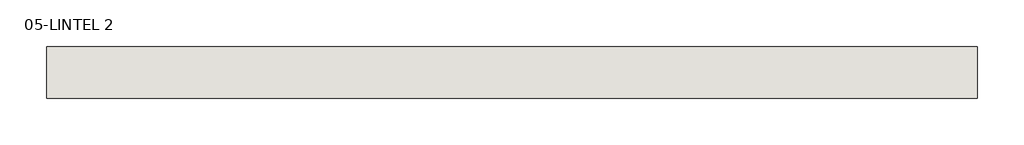
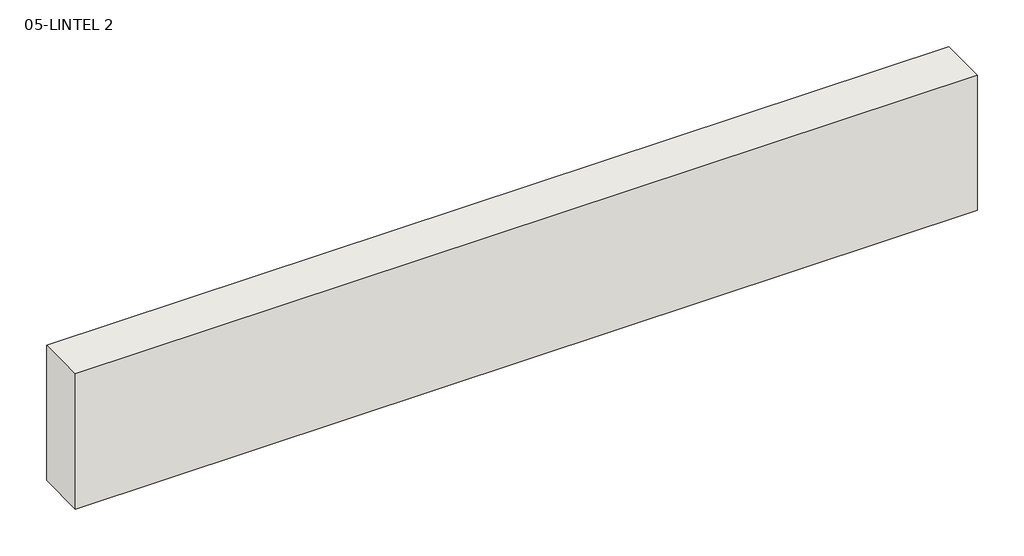
# One storey: 1 wall.
"""IFC4 building model written with IfcOpenShell, lengths in millimetres."""

from ifc_helpers import new_model, si_unit, frame, origin, place, context, project, spatial, polyline, outline, extrude, element, save

model = new_model("IFC4")

# Units and contexts
model_context = context("Model", 3, world=origin())
ifc_project = project(units=[si_unit("LENGTHUNIT", "METRE", prefix="MILLI")], contexts=[model_context])

# Site, building, storey
site = spatial("IfcSite", under=ifc_project)
building = spatial("IfcBuilding", under=site)
storey = spatial("IfcBuildingStorey", under=building, Name="05-LINTEL 2", Elevation=5850.0)

# Wall
placement = place(None, origin())
element("IfcWall", 1, ObjectType="01-225 WALL MAIN", at=placement, inside=storey, context=model_context, shape_type="SweptSolid", body=[
    extrude(outline(polyline([(-5642.6792561, -4186.7197682), (-9430.1792561, -4186.7197682), (-9430.1792561, -3976.7197682), (-5642.6792561, -3976.7197682), (-5642.6792561, -4186.7197682)])), frame((0.0, 0.0, 5850.0), z_axis=(0.0, 0.0, 1.0), x_axis=(1.0, 0.0, 0.0)), (0.0, 0.0, 1.0), 600.0),
])

save(model, "model.ifc")

# Revit data of these elements
# Type "01-225 WALL MAIN"
#   Description = "Generic Wall (Material By Category), 200mm thick"
#   Assembly Code = "B2010"
#   Type Mark = "G06"
#   Layers, outside or top first: 5 mm "01-WHITE WALL PAINT" (function 4); 200 mm "01-DEFAULT WALL" (function 1); 5 mm "01-WHITE WALL PAINT" (function 5)
# Element 1 (IfcWall, "01-225 WALL MAIN")
#   Top Offset = -300 mm
#   Base Offset = 0 mm
#   wall height = 600 mm
#   Phase Created = New Construction
#   Base Constraint = 05-LINTEL 2
#   Top Constraint = 06-CEILING
#   Materials on its faces: "Default Wall", "01-WHITE WALL PAINT"
# Materials
#   "01-WHITE WALL PAINT": class "Generic", colour RGB 242 242 255, transparency 0, Description = "Acoustic Ceiling Tile 24 x 48", Cost = 0
#   "01-DEFAULT WALL": class "Generic", colour RGB 242 242 255, transparency 0, Description = "Acoustic Ceiling Tile 24 x 48", Cost = 0
#   "Default Wall": colour RGB 192 192 192, transparency 0, Cost = 0
